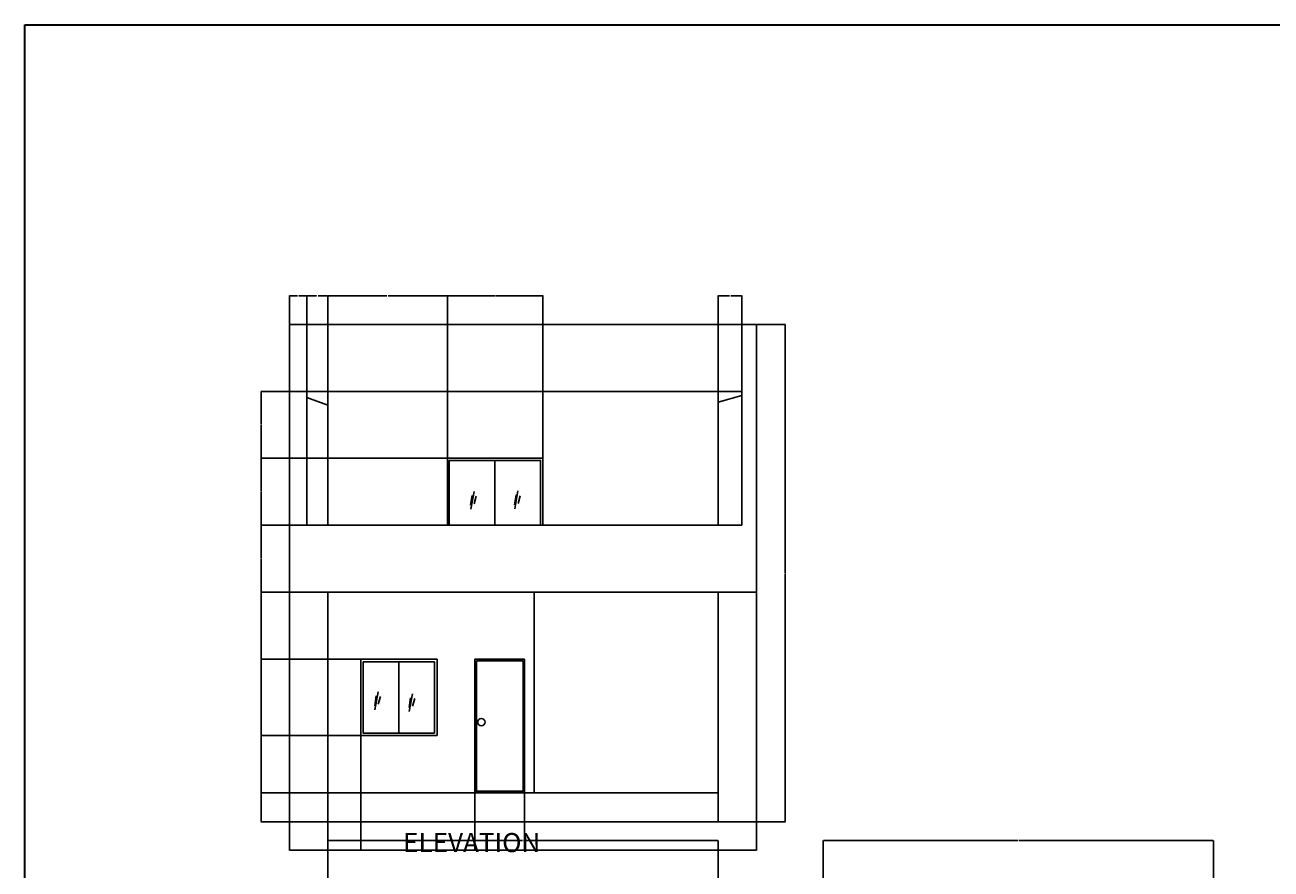
# Model space of a CAD drawing. Units: inches. Extents: x 1850 to 3445, y 1558 to 2756.
# Tile 8 of 13: x 1850 to 2632, y 2227 to 2756. Entities that reach past the tile are written whole.
import ezdxf

# ---------------------------------------------------------------- set-up
doc = ezdxf.new("R2010")
doc.units = ezdxf.units.IN
for name, color, linetype, lineweight in [('A-ANNO-DIMS', 2, 'Continuous', 18), ('A-ANNO-TEXT', 7, 'Continuous', 18), ('A-ANNO-TTLB', 7, 'Continuous', 35), ('A-ELEV', 7, 'Continuous', 25)]:
    doc.layers.add(name, color=color, linetype=linetype, lineweight=lineweight)
doc.styles.get("Standard").update_dxf_attribs({"font": 'arial.ttf'})
doc.dimstyles.get("Standard").update_dxf_attribs({"dimtxt": 0.18, "dimasz": 0.18, "dimexe": 0.18, "dimexo": 0.0625, "dimgap": 0.09, "dimtad": 0, "dimtih": 1, "dimtoh": 1, "dimdec": 4, "dimzin": 0, "dimdsep": 46, "dimtxsty": 'Standard', "dimcen": 0.09, "dimadec": 0, "dimazin": 0, "dimtfac": 1, "dimtdec": 4, "dimtofl": 0, "dimtmove": 0, "dimatfit": 3, "dimfxl": 1, "dimtolj": 1, "dimtzin": 0, "dimarcsym": 0})

# ---------------------------------------------------------------- blocks, each defined once
blk = doc.blocks.new('GLASS-REFLECTION')
for p, q in [((0.97, 8.75), (0, 2.61)), ((2.14, 11.25), (0.13, 0)), ((3.57, 8.31), (2.19, 3.48))]:
    blk.add_line(p, q)
blk = doc.blocks.new('*D80')
at = {"layer": 'A-ANNO-DIMS', "color": 0, "lineweight": -2, "transparency": 16777216}
for p, q in [((2040.27, 2216.25), (2040.27, 2244.61)), ((2040.45, 2244.43), (2162.48, 2244.43)), ((2285.09, 2244.43), (2163.06, 2244.43)), ((2285.27, 2216.25), (2285.27, 2244.61))]:
    blk.add_line(p, q, dxfattribs=at)
at = {"layer": 'A-ANNO-DIMS', "color": 0, "transparency": 16777216}
for points in [[(2040.45, 2244.46), (2040.45, 2244.4), (2040.27, 2244.43)], [(2285.09, 2244.46), (2285.09, 2244.4), (2285.27, 2244.43)]]:
    blk.add_solid(points, dxfattribs=at)
at = {"layer": 'Defpoints', "color": 0, "transparency": 16777216}
for p in [(2285.27, 2244.43), (2040.27, 2216.18), (2285.27, 2216.18)]:
    blk.add_point(p, dxfattribs=at)
at = {"layer": 'A-ANNO-DIMS', "color": 0, "transparency": 16777216, "insert": (2162.77, 2244.43), "char_height": 0.18, "attachment_point": 5}
blk.add_mtext('\\A1;245', dxfattribs=at)
blk = doc.blocks.new('*D82')
at = {"layer": 'A-ANNO-DIMS', "color": 0, "lineweight": -2, "transparency": 16777216}
for p, q in [((2351.06, 2216.25), (2351.06, 2244.61)), ((2351.24, 2244.43), (2473.26, 2244.43)), ((2595.88, 2244.43), (2473.85, 2244.43)), ((2596.06, 2216.25), (2596.06, 2244.61))]:
    blk.add_line(p, q, dxfattribs=at)
at = {"layer": 'A-ANNO-DIMS', "color": 0, "transparency": 16777216}
for points in [[(2351.24, 2244.46), (2351.24, 2244.4), (2351.06, 2244.43)], [(2595.88, 2244.46), (2595.88, 2244.4), (2596.06, 2244.43)]]:
    blk.add_solid(points, dxfattribs=at)
at = {"layer": 'Defpoints', "color": 0, "transparency": 16777216}
for p in [(2596.06, 2244.43), (2351.06, 2216.18), (2596.06, 2216.18)]:
    blk.add_point(p, dxfattribs=at)
at = {"layer": 'A-ANNO-DIMS', "color": 0, "transparency": 16777216, "insert": (2473.56, 2244.43), "char_height": 0.18, "attachment_point": 5}
blk.add_mtext('\\A1;245', dxfattribs=at)
blk = doc.blocks.new('*D106')
at = {"layer": 'A-ANNO-DIMS', "color": 0, "lineweight": -2, "transparency": 16777216}
for p, q in [((2016.27, 2400.29), (2016.27, 2238.24)), ((2309.27, 2400.29), (2309.27, 2238.24)), ((2016.45, 2238.42), (2162.48, 2238.42)), ((2309.09, 2238.42), (2163.06, 2238.42))]:
    blk.add_line(p, q, dxfattribs=at)
at = {"layer": 'A-ANNO-DIMS', "color": 0, "transparency": 16777216}
for points in [[(2016.45, 2238.45), (2016.45, 2238.39), (2016.27, 2238.42)], [(2309.09, 2238.45), (2309.09, 2238.39), (2309.27, 2238.42)]]:
    blk.add_solid(points, dxfattribs=at)
at = {"layer": 'Defpoints', "color": 0, "transparency": 16777216}
for p in [(2016.27, 2400.35), (2309.27, 2400.35), (2309.27, 2238.42)]:
    blk.add_point(p, dxfattribs=at)
at = {"layer": 'A-ANNO-DIMS', "color": 0, "transparency": 16777216, "insert": (2162.77, 2238.42), "char_height": 0.18, "attachment_point": 5}
blk.add_mtext('\\A1;293', dxfattribs=at)
blk = doc.blocks.new('*D107')
at = {"layer": 'A-ANNO-DIMS', "color": 0, "lineweight": -2, "transparency": 16777216}
for p, q in [((2309.33, 2568.35), (2327.38, 2568.35)), ((2327.2, 2568.17), (2327.2, 2412.53)), ((2327.2, 2256.53), (2327.2, 2412.17)), ((2285.33, 2256.35), (2327.38, 2256.35))]:
    blk.add_line(p, q, dxfattribs=at)
at = {"layer": 'A-ANNO-DIMS', "color": 0, "transparency": 16777216}
for points in [[(2327.17, 2568.17), (2327.23, 2568.17), (2327.2, 2568.35)], [(2327.17, 2256.53), (2327.23, 2256.53), (2327.2, 2256.35)]]:
    blk.add_solid(points, dxfattribs=at)
at = {"layer": 'Defpoints', "color": 0, "transparency": 16777216}
for p in [(2309.27, 2568.35), (2327.2, 2568.35), (2285.27, 2256.35)]:
    blk.add_point(p, dxfattribs=at)
at = {"layer": 'A-ANNO-DIMS', "color": 0, "transparency": 16777216, "insert": (2327.2, 2412.35), "char_height": 0.18, "attachment_point": 5}
blk.add_mtext('\\A1;312', dxfattribs=at)
blk = doc.blocks.new('*D108')
at = {"layer": 'A-ANNO-DIMS', "color": 0, "lineweight": -2, "transparency": 16777216}
for p, q in [((2040.21, 2274.35), (1998.17, 2274.35)), ((1998.35, 2274.17), (1998.35, 2265.53)), ((1998.35, 2256.53), (1998.35, 2265.17)), ((2040.21, 2256.35), (1998.17, 2256.35))]:
    blk.add_line(p, q, dxfattribs=at)
at = {"layer": 'A-ANNO-DIMS', "color": 0, "transparency": 16777216}
for points in [[(1998.32, 2274.17), (1998.38, 2274.17), (1998.35, 2274.35)], [(1998.32, 2256.53), (1998.38, 2256.53), (1998.35, 2256.35)]]:
    blk.add_solid(points, dxfattribs=at)
at = {"layer": 'Defpoints', "color": 0, "transparency": 16777216}
for p in [(1998.35, 2274.35), (2040.27, 2274.35), (2040.27, 2256.35)]:
    blk.add_point(p, dxfattribs=at)
at = {"layer": 'A-ANNO-DIMS', "color": 0, "transparency": 16777216, "insert": (1998.35, 2265.35), "char_height": 0.18, "attachment_point": 5}
blk.add_mtext('\\A1;18', dxfattribs=at)
blk = doc.blocks.new('*D109')
at = {"layer": 'A-ANNO-DIMS', "color": 0, "lineweight": -2, "transparency": 16777216}
for p, q in [((2060.89, 2310.35), (1998.17, 2310.35)), ((1998.35, 2310.17), (1998.35, 2292.53)), ((1998.35, 2274.53), (1998.35, 2292.17)), ((2040.21, 2274.35), (1998.17, 2274.35))]:
    blk.add_line(p, q, dxfattribs=at)
at = {"layer": 'A-ANNO-DIMS', "color": 0, "transparency": 16777216}
for points in [[(1998.32, 2310.17), (1998.38, 2310.17), (1998.35, 2310.35)], [(1998.32, 2274.53), (1998.38, 2274.53), (1998.35, 2274.35)]]:
    blk.add_solid(points, dxfattribs=at)
at = {"layer": 'Defpoints', "color": 0, "transparency": 16777216}
for p in [(1998.35, 2310.35), (2060.95, 2310.35), (2040.27, 2274.35)]:
    blk.add_point(p, dxfattribs=at)
at = {"layer": 'A-ANNO-DIMS', "color": 0, "transparency": 16777216, "insert": (1998.35, 2292.35), "char_height": 0.18, "attachment_point": 5}
blk.add_mtext('\\A1;36', dxfattribs=at)
blk = doc.blocks.new('*D110')
at = {"layer": 'A-ANNO-DIMS', "color": 0, "lineweight": -2, "transparency": 16777216}
for p, q in [((2060.89, 2358.35), (1998.17, 2358.35)), ((1998.35, 2358.17), (1998.35, 2334.53)), ((1998.35, 2310.53), (1998.35, 2334.17)), ((2060.89, 2310.35), (1998.17, 2310.35))]:
    blk.add_line(p, q, dxfattribs=at)
at = {"layer": 'A-ANNO-DIMS', "color": 0, "transparency": 16777216}
for points in [[(1998.32, 2358.17), (1998.38, 2358.17), (1998.35, 2358.35)], [(1998.32, 2310.53), (1998.38, 2310.53), (1998.35, 2310.35)]]:
    blk.add_solid(points, dxfattribs=at)
at = {"layer": 'Defpoints', "color": 0, "transparency": 16777216}
for p in [(1998.35, 2358.35), (2060.95, 2358.35), (2060.95, 2310.35)]:
    blk.add_point(p, dxfattribs=at)
at = {"layer": 'A-ANNO-DIMS', "color": 0, "transparency": 16777216, "insert": (1998.35, 2334.35), "char_height": 0.18, "attachment_point": 5}
blk.add_mtext('\\A1;48', dxfattribs=at)
blk = doc.blocks.new('*D111')
at = {"layer": 'A-ANNO-DIMS', "color": 0, "lineweight": -2, "transparency": 16777216}
for p, q in [((2040.21, 2400.35), (1998.17, 2400.35)), ((1998.35, 2400.17), (1998.35, 2379.53)), ((1998.35, 2358.53), (1998.35, 2379.17)), ((2060.89, 2358.35), (1998.17, 2358.35))]:
    blk.add_line(p, q, dxfattribs=at)
at = {"layer": 'A-ANNO-DIMS', "color": 0, "transparency": 16777216}
for points in [[(1998.32, 2400.17), (1998.38, 2400.17), (1998.35, 2400.35)], [(1998.32, 2358.53), (1998.38, 2358.53), (1998.35, 2358.35)]]:
    blk.add_solid(points, dxfattribs=at)
at = {"layer": 'Defpoints', "color": 0, "transparency": 16777216}
for p in [(1998.35, 2400.35), (2040.27, 2400.35), (2060.95, 2358.35)]:
    blk.add_point(p, dxfattribs=at)
at = {"layer": 'A-ANNO-DIMS', "color": 0, "transparency": 16777216, "insert": (1998.35, 2379.35), "char_height": 0.18, "attachment_point": 5}
blk.add_mtext('\\A1;42', dxfattribs=at)
blk = doc.blocks.new('*D112')
at = {"layer": 'A-ANNO-DIMS', "color": 0, "lineweight": -2, "transparency": 16777216}
for p, q in [((2026.99, 2442.35), (1998.17, 2442.35)), ((1998.35, 2442.17), (1998.35, 2421.53)), ((1998.35, 2400.53), (1998.35, 2421.17)), ((2016.21, 2400.35), (1998.17, 2400.35))]:
    blk.add_line(p, q, dxfattribs=at)
at = {"layer": 'A-ANNO-DIMS', "color": 0, "transparency": 16777216}
for points in [[(1998.32, 2442.17), (1998.38, 2442.17), (1998.35, 2442.35)], [(1998.32, 2400.53), (1998.38, 2400.53), (1998.35, 2400.35)]]:
    blk.add_solid(points, dxfattribs=at)
at = {"layer": 'Defpoints', "color": 0, "transparency": 16777216}
for p in [(1998.35, 2442.35), (2027.05, 2442.35), (2016.27, 2400.35)]:
    blk.add_point(p, dxfattribs=at)
at = {"layer": 'A-ANNO-DIMS', "color": 0, "transparency": 16777216, "insert": (1998.35, 2421.35), "char_height": 0.18, "attachment_point": 5}
blk.add_mtext('\\A1;42', dxfattribs=at)
blk = doc.blocks.new('*D113')
at = {"layer": 'A-ANNO-DIMS', "color": 0, "lineweight": -2, "transparency": 16777216}
for p, q in [((2115.19, 2484.35), (1998.17, 2484.35)), ((1998.35, 2484.17), (1998.35, 2463.53)), ((1998.35, 2442.53), (1998.35, 2463.17)), ((2026.99, 2442.35), (1998.17, 2442.35))]:
    blk.add_line(p, q, dxfattribs=at)
at = {"layer": 'A-ANNO-DIMS', "color": 0, "transparency": 16777216}
for points in [[(1998.32, 2484.17), (1998.38, 2484.17), (1998.35, 2484.35)], [(1998.32, 2442.53), (1998.38, 2442.53), (1998.35, 2442.35)]]:
    blk.add_solid(points, dxfattribs=at)
at = {"layer": 'Defpoints', "color": 0, "transparency": 16777216}
for p in [(1998.35, 2484.35), (2115.25, 2484.35), (2027.05, 2442.35)]:
    blk.add_point(p, dxfattribs=at)
at = {"layer": 'A-ANNO-DIMS', "color": 0, "transparency": 16777216, "insert": (1998.35, 2463.35), "char_height": 0.18, "attachment_point": 5}
blk.add_mtext('\\A1;42', dxfattribs=at)
blk = doc.blocks.new('*D114')
at = {"layer": 'A-ANNO-DIMS', "color": 0, "lineweight": -2, "transparency": 16777216}
for p, q in [((2026.99, 2526.35), (1998.17, 2526.35)), ((1998.35, 2526.17), (1998.35, 2505.53)), ((1998.35, 2484.53), (1998.35, 2505.17)), ((2115.19, 2484.35), (1998.17, 2484.35))]:
    blk.add_line(p, q, dxfattribs=at)
at = {"layer": 'A-ANNO-DIMS', "color": 0, "transparency": 16777216}
for points in [[(1998.32, 2526.17), (1998.38, 2526.17), (1998.35, 2526.35)], [(1998.32, 2484.53), (1998.38, 2484.53), (1998.35, 2484.35)]]:
    blk.add_solid(points, dxfattribs=at)
at = {"layer": 'Defpoints', "color": 0, "transparency": 16777216}
for p in [(1998.35, 2526.35), (2027.05, 2526.35), (2115.25, 2484.35)]:
    blk.add_point(p, dxfattribs=at)
at = {"layer": 'A-ANNO-DIMS', "color": 0, "transparency": 16777216, "insert": (1998.35, 2505.35), "char_height": 0.18, "attachment_point": 5}
blk.add_mtext('\\A1;42', dxfattribs=at)
blk = doc.blocks.new('*D115')
at = {"layer": 'A-ANNO-DIMS', "color": 0, "lineweight": -2, "transparency": 16777216}
for p, q in [((2060.95, 2310.29), (2060.95, 2238.24)), ((2040.27, 2256.29), (2040.27, 2238.24)), ((2040.45, 2238.42), (2050.14, 2238.42)), ((2060.77, 2238.42), (2051.07, 2238.42))]:
    blk.add_line(p, q, dxfattribs=at)
at = {"layer": 'A-ANNO-DIMS', "color": 0, "transparency": 16777216}
for points in [[(2040.45, 2238.45), (2040.45, 2238.39), (2040.27, 2238.42)], [(2060.77, 2238.45), (2060.77, 2238.39), (2060.95, 2238.42)]]:
    blk.add_solid(points, dxfattribs=at)
at = {"layer": 'Defpoints', "color": 0, "transparency": 16777216}
for p in [(2060.95, 2310.35), (2040.27, 2256.35), (2060.95, 2238.42)]:
    blk.add_point(p, dxfattribs=at)
at = {"layer": 'A-ANNO-DIMS', "color": 0, "transparency": 16777216, "insert": (2050.61, 2238.42), "char_height": 0.18, "attachment_point": 5}
blk.add_mtext('\\A1;20.677', dxfattribs=at)
blk = doc.blocks.new('*D116')
at = {"layer": 'A-ANNO-DIMS', "color": 0, "lineweight": -2, "transparency": 16777216}
for p, q in [((2132.49, 2274.29), (2132.49, 2238.24)), ((2163.69, 2274.29), (2163.69, 2238.24)), ((2132.67, 2238.42), (2147.63, 2238.42)), ((2163.51, 2238.42), (2148.55, 2238.42))]:
    blk.add_line(p, q, dxfattribs=at)
at = {"layer": 'A-ANNO-DIMS', "color": 0, "transparency": 16777216}
for points in [[(2132.67, 2238.45), (2132.67, 2238.39), (2132.49, 2238.42)], [(2163.51, 2238.45), (2163.51, 2238.39), (2163.69, 2238.42)]]:
    blk.add_solid(points, dxfattribs=at)
at = {"layer": 'Defpoints', "color": 0, "transparency": 16777216}
for p in [(2132.49, 2274.35), (2163.69, 2274.35), (2163.69, 2238.42)]:
    blk.add_point(p, dxfattribs=at)
at = {"layer": 'A-ANNO-DIMS', "color": 0, "transparency": 16777216, "insert": (2148.09, 2238.42), "char_height": 0.18, "attachment_point": 5}
blk.add_mtext('\\A1;31.193', dxfattribs=at)
blk = doc.blocks.new('*D117')
at = {"layer": 'A-ANNO-DIMS', "color": 0, "lineweight": -2, "transparency": 16777216}
for p, q in [((2016.27, 2568.41), (2016.27, 2586.45)), ((2016.45, 2586.27), (2021.2, 2586.27)), ((2026.87, 2586.27), (2022.12, 2586.27)), ((2027.05, 2526.41), (2027.05, 2586.45))]:
    blk.add_line(p, q, dxfattribs=at)
at = {"layer": 'A-ANNO-DIMS', "color": 0, "transparency": 16777216}
for points in [[(2016.45, 2586.3), (2016.45, 2586.24), (2016.27, 2586.27)], [(2026.87, 2586.3), (2026.87, 2586.24), (2027.05, 2586.27)]]:
    blk.add_solid(points, dxfattribs=at)
at = {"layer": 'Defpoints', "color": 0, "transparency": 16777216}
for p in [(2027.05, 2586.27), (2016.27, 2568.35), (2027.05, 2526.35)]:
    blk.add_point(p, dxfattribs=at)
at = {"layer": 'A-ANNO-DIMS', "color": 0, "transparency": 16777216, "insert": (2021.66, 2586.27), "char_height": 0.18, "attachment_point": 5}
blk.add_mtext('\\A1;10.777', dxfattribs=at)
blk = doc.blocks.new('*D118')
at = {"layer": 'A-ANNO-DIMS', "color": 0, "lineweight": -2, "transparency": 16777216}
for p, q in [((2027.05, 2526.41), (2027.05, 2586.45)), ((2027.23, 2586.27), (2033.2, 2586.27)), ((2040.09, 2586.27), (2034.12, 2586.27)), ((2040.27, 2526.41), (2040.27, 2586.45))]:
    blk.add_line(p, q, dxfattribs=at)
at = {"layer": 'A-ANNO-DIMS', "color": 0, "transparency": 16777216}
for points in [[(2027.23, 2586.3), (2027.23, 2586.24), (2027.05, 2586.27)], [(2040.09, 2586.3), (2040.09, 2586.24), (2040.27, 2586.27)]]:
    blk.add_solid(points, dxfattribs=at)
at = {"layer": 'Defpoints', "color": 0, "transparency": 16777216}
for p in [(2040.27, 2586.27), (2027.05, 2526.35), (2040.27, 2526.35)]:
    blk.add_point(p, dxfattribs=at)
at = {"layer": 'A-ANNO-DIMS', "color": 0, "transparency": 16777216, "insert": (2033.66, 2586.27), "char_height": 0.18, "attachment_point": 5}
blk.add_mtext('\\A1;13.223', dxfattribs=at)
blk = doc.blocks.new('*D119')
at = {"layer": 'A-ANNO-DIMS', "color": 0, "lineweight": -2, "transparency": 16777216}
for p, q in [((2040.27, 2526.41), (2040.27, 2586.45)), ((2040.45, 2586.27), (2077.37, 2586.27)), ((2115.07, 2586.27), (2078.15, 2586.27)), ((2115.25, 2484.41), (2115.25, 2586.45))]:
    blk.add_line(p, q, dxfattribs=at)
at = {"layer": 'A-ANNO-DIMS', "color": 0, "transparency": 16777216}
for points in [[(2040.45, 2586.3), (2040.45, 2586.24), (2040.27, 2586.27)], [(2115.07, 2586.3), (2115.07, 2586.24), (2115.25, 2586.27)]]:
    blk.add_solid(points, dxfattribs=at)
at = {"layer": 'Defpoints', "color": 0, "transparency": 16777216}
for p in [(2115.25, 2586.27), (2040.27, 2526.35), (2115.25, 2484.35)]:
    blk.add_point(p, dxfattribs=at)
at = {"layer": 'A-ANNO-DIMS', "color": 0, "transparency": 16777216, "insert": (2077.76, 2586.27), "char_height": 0.18, "attachment_point": 5}
blk.add_mtext('\\A1;74.98', dxfattribs=at)
blk = doc.blocks.new('*D120')
at = {"layer": 'A-ANNO-DIMS', "color": 0, "lineweight": -2, "transparency": 16777216}
for p, q in [((2115.25, 2484.41), (2115.25, 2586.45)), ((2115.43, 2586.27), (2145.03, 2586.27)), ((2175.07, 2586.27), (2145.47, 2586.27)), ((2175.25, 2484.41), (2175.25, 2586.45))]:
    blk.add_line(p, q, dxfattribs=at)
at = {"layer": 'A-ANNO-DIMS', "color": 0, "transparency": 16777216}
for points in [[(2115.43, 2586.3), (2115.43, 2586.24), (2115.25, 2586.27)], [(2175.07, 2586.3), (2175.07, 2586.24), (2175.25, 2586.27)]]:
    blk.add_solid(points, dxfattribs=at)
at = {"layer": 'Defpoints', "color": 0, "transparency": 16777216}
for p in [(2175.25, 2586.27), (2115.25, 2484.35), (2175.25, 2484.35)]:
    blk.add_point(p, dxfattribs=at)
at = {"layer": 'A-ANNO-DIMS', "color": 0, "transparency": 16777216, "insert": (2145.25, 2586.27), "char_height": 0.18, "attachment_point": 5}
blk.add_mtext('\\A1;60', dxfattribs=at)
blk = doc.blocks.new('*D121')
at = {"layer": 'A-ANNO-DIMS', "color": 0, "lineweight": -2, "transparency": 16777216}
for p, q in [((2285.27, 2526.41), (2285.27, 2586.45)), ((2285.45, 2586.27), (2292.22, 2586.27)), ((2299.9, 2586.27), (2293.13, 2586.27)), ((2300.08, 2526.41), (2300.08, 2586.45))]:
    blk.add_line(p, q, dxfattribs=at)
at = {"layer": 'A-ANNO-DIMS', "color": 0, "transparency": 16777216}
for points in [[(2285.45, 2586.3), (2285.45, 2586.24), (2285.27, 2586.27)], [(2299.9, 2586.3), (2299.9, 2586.24), (2300.08, 2586.27)]]:
    blk.add_solid(points, dxfattribs=at)
at = {"layer": 'Defpoints', "color": 0, "transparency": 16777216}
for p in [(2300.08, 2586.27), (2285.27, 2526.35), (2300.08, 2526.35)]:
    blk.add_point(p, dxfattribs=at)
at = {"layer": 'A-ANNO-DIMS', "color": 0, "transparency": 16777216, "insert": (2292.68, 2586.27), "char_height": 0.18, "attachment_point": 5}
blk.add_mtext('\\A1;14.812', dxfattribs=at)

msp = doc.modelspace()

# ---------------------------------------------------------------- linework, layer by layer
at = {"layer": 'A-ANNO-TTLB'}
msp.add_lwpolyline([(1850.1793, 2756.3177), (3445.2682, 2756.3177), (3445.2682, 1557.7728), (1850.1793, 1557.7728)], close=True, dxfattribs=at)
at = {"layer": 'A-ELEV'}
for p, q in [((2309.2715, 2568.3497), (2016.2715, 2568.3497)), ((2016.2715, 2526.3497), (2016.2715, 2568.3497)), ((2309.2715, 2526.3497), (2309.2715, 2568.3497)), ((2016.2715, 2526.3497), (2016.2715, 2442.3497)), ((2300.0836, 2526.3497), (2027.0483, 2526.3497)), ((2027.0483, 2526.3497), (2027.0483, 2442.3497)), ((2040.2715, 2526.3497), (2040.2715, 2442.3497)), ((2285.2715, 2526.3497), (2285.2715, 2442.3497)), ((2300.0836, 2526.3497), (2300.0836, 2442.3497)), ((2309.2715, 2526.3497), (2309.2715, 2442.3497)), ((2027.0483, 2522.4553), (2040.2715, 2517.6768)), ((2300.0836, 2523.7826), (2285.2715, 2519.6442)), ((2115.2489, 2484.3497), (2115.2489, 2442.3497)), ((2175.2489, 2484.3497), (2115.2489, 2484.3497)), ((2145.095, 2483.0443), (2145.095, 2442.3497)), ((2175.2489, 2484.3497), (2175.2489, 2442.3497)), ((2016.2715, 2400.3497), (2016.2715, 2442.3497)), ((2300.0836, 2442.3497), (2027.0483, 2442.3497)), ((2309.2715, 2400.3497), (2309.2715, 2442.3497)), ((2309.2715, 2400.3497), (2016.2715, 2400.3497)), ((2040.2715, 2400.3497), (2040.2715, 2256.3497)), ((2040.2715, 2400.3497), (2040.2715, 2382.3497)), ((2169.7715, 2400.3497), (2169.7715, 2274.3497)), ((2285.2715, 2400.3497), (2285.2715, 2256.3497)), ((2285.2715, 2400.3497), (2285.2715, 2382.3497)), ((2060.9481, 2358.3497), (2060.9481, 2310.3497)), ((2108.9481, 2358.3497), (2060.9481, 2358.3497)), ((2084.7483, 2356.6236), (2084.7483, 2311.9749)), ((2108.9481, 2358.3497), (2108.9481, 2310.3497)), ((2132.4938, 2358.3497), (2132.4938, 2274.3497)), ((2163.687, 2358.3497), (2132.4938, 2358.3497)), ((2163.687, 2358.3497), (2163.687, 2274.3497)), ((2108.9481, 2310.3497), (2060.9481, 2310.3497)), ((2285.2715, 2274.3497), (2040.2715, 2274.3497)), ((2285.2715, 2256.3497), (2040.2715, 2256.3497))]:
    msp.add_line(p, q, dxfattribs=at)
msp.add_lwpolyline([(2116.4446, 2442.3497), (2116.4446, 2483.0443), (2173.7454, 2483.0443), (2173.7454, 2442.3497)], dxfattribs=at)
for points in [[(2062.3573, 2356.6236), (2107.1392, 2356.6236), (2107.1392, 2311.9749), (2062.3573, 2311.9749)], [(2133.5044, 2357.2133), (2162.7512, 2357.2133), (2162.7512, 2275.396), (2133.5044, 2275.396)]]:
    msp.add_lwpolyline(points, close=True, dxfattribs=at)
msp.add_circle((2136.5978, 2318.8277), 2.292, dxfattribs=at)

# ---------------------------------------------------------------- block references
for p in [(2129.8479, 2452.3474), (2157.413, 2452.6), (2069.651, 2326.5217), (2091.252, 2325.3782)]:
    msp.add_blockref('GLASS-REFLECTION', p, dxfattribs=at)

# ---------------------------------------------------------------- texts
at = {"layer": 'A-ANNO-TEXT', "insert": (2087.5055, 2249.2282), "char_height": 12, "attachment_point": 1}
msp.add_mtext_dynamic_manual_height_columns('ELEVATION', width=229.740704, gutter_width=12.5, heights=[0], dxfattribs=at)

# ---------------------------------------------------------------- dimensions: what is measured, and where the dimension line sits
at = {"layer": 'A-ANNO-DIMS'}
for base, p1, p2, override, picture, middle in [((2027.0483, 2586.2747), (2016.2715, 2568.3497), (2027.0483, 2526.3497), {"dimdec": 3, "dimlfac": 1, "dimrnd": 0, "dimzin": 0, "dimdsep": 46, "dimlunit": 2}, '*D117', (2021.6599, 2586.2747)), ((2040.2715, 2586.2747), (2027.0483, 2526.3497), (2040.2715, 2526.3497), {"dimdec": 3, "dimlfac": 1, "dimrnd": 0, "dimzin": 0, "dimdsep": 46, "dimlunit": 2}, '*D118', (2033.6599, 2586.2747)), ((2115.2489, 2586.2747), (2040.2715, 2526.3497), (2115.2489, 2484.3497), {"dimdec": 2, "dimlfac": 1, "dimrnd": 0, "dimzin": 0, "dimdsep": 46, "dimlunit": 2}, '*D119', (2077.7602, 2586.2747)), ((2175.2489, 2586.2747), (2115.2489, 2484.3497), (2175.2489, 2484.3497), {"dimdec": 0, "dimlfac": 1, "dimrnd": 0, "dimzin": 0, "dimdsep": 46, "dimlunit": 2}, '*D120', (2145.2489, 2586.2747)), ((2300.0836, 2586.2747), (2285.2715, 2526.3497), (2300.0836, 2526.3497), {"dimdec": 3, "dimlfac": 1, "dimrnd": 0, "dimzin": 0, "dimdsep": 46, "dimlunit": 2}, '*D121', (2292.6775, 2586.2747)), ((2309.2715, 2238.4247), (2016.2715, 2400.3497), (2309.2715, 2400.3497), {"dimdec": 0, "dimlfac": 1, "dimrnd": 0, "dimzin": 0, "dimdsep": 46, "dimlunit": 2}, '*D106', (2162.7715, 2238.4247)), ((2060.9481, 2238.4247), (2040.2715, 2256.3497), (2060.9481, 2310.3497), {"dimdec": 3, "dimlfac": 1, "dimrnd": 0, "dimzin": 0, "dimdsep": 46, "dimlunit": 2}, '*D115', (2050.6098, 2238.4247)), ((2163.687, 2238.4247), (2132.4938, 2274.3497), (2163.687, 2274.3497), {"dimdec": 3, "dimlfac": 1, "dimrnd": 0, "dimzin": 0, "dimdsep": 46, "dimlunit": 2}, '*D116', (2148.0904, 2238.4247)), ((2285.2715, 2244.4343), (2040.2715, 2216.1843), (2285.2715, 2216.1843), {"dimdec": 0, "dimlfac": 1, "dimrnd": 0, "dimzin": 0, "dimdsep": 46, "dimlunit": 2}, '*D80', (2162.7715, 2244.4343)), ((2596.0556, 2244.4343), (2351.0556, 2216.1843), (2596.0556, 2216.1843), {"dimdec": 0, "dimlfac": 1, "dimrnd": 0, "dimzin": 0, "dimdsep": 46, "dimlunit": 2}, '*D82', (2473.5556, 2244.4343))]:
    dim = msp.add_linear_dim(base=base, p1=p1, p2=p2, dimstyle='Standard', override=override, dxfattribs=at)
    dim.commit()
    dim.dimension.update_dxf_attribs({"geometry": picture, "text_midpoint": middle})
for base, p1, p2, picture, middle in [((2327.1965, 2568.3497), (2285.2715, 2256.3497), (2309.2715, 2568.3497), '*D107', (2327.1965, 2412.3497)), ((1998.3465, 2526.3497), (2115.2489, 2484.3497), (2027.0483, 2526.3497), '*D114', (1998.3465, 2505.3497)), ((1998.3465, 2484.3497), (2027.0483, 2442.3497), (2115.2489, 2484.3497), '*D113', (1998.3465, 2463.3497)), ((1998.3465, 2442.3497), (2016.2715, 2400.3497), (2027.0483, 2442.3497), '*D112', (1998.3465, 2421.3497)), ((1998.3465, 2400.3497), (2060.9481, 2358.3497), (2040.2715, 2400.3497), '*D111', (1998.3465, 2379.3497)), ((1998.3465, 2358.3497), (2060.9481, 2310.3497), (2060.9481, 2358.3497), '*D110', (1998.3465, 2334.3497)), ((1998.3465, 2310.3497), (2040.2715, 2274.3497), (2060.9481, 2310.3497), '*D109', (1998.3465, 2292.3497)), ((1998.3465, 2274.3497), (2040.2715, 2256.3497), (2040.2715, 2274.3497), '*D108', (1998.3465, 2265.3497))]:
    dim = msp.add_linear_dim(base=base, p1=p1, p2=p2, angle=90, dimstyle='Standard', override={"dimdec": 0, "dimlfac": 1, "dimrnd": 0, "dimzin": 0, "dimdsep": 46, "dimlunit": 2}, dxfattribs=at)
    dim.commit()
    dim.dimension.update_dxf_attribs({"geometry": picture, "text_midpoint": middle})

doc.saveas('drawing.dxf')
